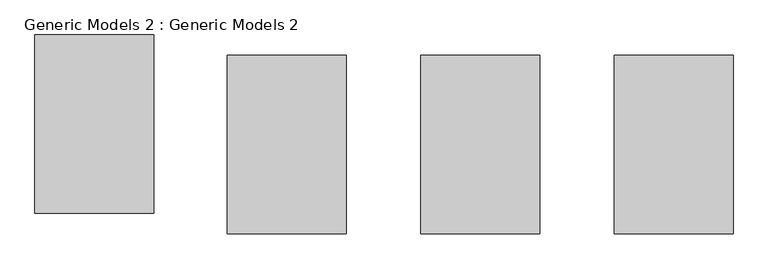
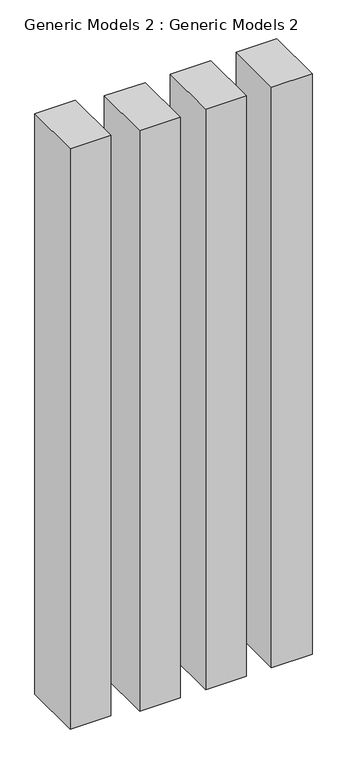
"""IFC4 building model written with IfcOpenShell, lengths in millimetres: proxy geometry, Generic Models 2 : Generic Models 2."""

from ifc_helpers import new_model, si_unit, frame, origin, place, context, project, spatial, polyline, outline, extrude, source, transform, mapped, element, save


def generic_models_2_generic_models_2_13199aed(model_context):
    return source(origin(), model_context, "Body", "SweptSolid", [
        extrude(outline(polyline([(-5406.6672301, -7265.2302427), (-5203.4672301, -7265.2302427), (-5203.4672301, -7570.0302427), (-5406.6672301, -7570.0302427), (-5406.6672301, -7265.2302427)])), frame((0.0, 0.0, 3022.6), z_axis=(0.0, 0.0, 1.0), x_axis=(1.0, 0.0, 0.0)), (0.0, 0.0, 1.0), 3073.4),
        extrude(outline(polyline([(-5736.8672301, -7265.2302427), (-5533.6672301, -7265.2302427), (-5533.6672301, -7570.0302427), (-5736.8672301, -7570.0302427), (-5736.8672301, -7265.2302427)])), frame((0.0, 0.0, 3022.6), z_axis=(0.0, 0.0, 1.0), x_axis=(1.0, 0.0, 0.0)), (0.0, 0.0, 1.0), 3073.4),
        extrude(outline(polyline([(-6067.0672301, -7265.2302427), (-5863.8672301, -7265.2302427), (-5863.8672301, -7570.0302427), (-6067.0672301, -7570.0302427), (-6067.0672301, -7265.2302427)])), frame((0.0, 0.0, 3022.6), z_axis=(0.0, 0.0, 1.0), x_axis=(1.0, 0.0, 0.0)), (0.0, 0.0, 1.0), 3073.4),
        extrude(outline(polyline([(-6395.45836, -7230.7149442), (-6192.25836, -7230.7149442), (-6192.25836, -7535.5149442), (-6395.45836, -7535.5149442), (-6395.45836, -7230.7149442)])), frame((0.0, 0.0, 3022.6), z_axis=(0.0, 0.0, 1.0), x_axis=(1.0, 0.0, 0.0)), (0.0, 0.0, 1.0), 3073.4),
    ])


if __name__ == "__main__":
    model = new_model("IFC4")
    model_context = context("Model", 3, world=origin())
    ifc_project = project(units=[si_unit("LENGTHUNIT", "METRE", prefix="MILLI")], contexts=[model_context])
    site = spatial("IfcSite", under=ifc_project)
    building = spatial("IfcBuilding", under=site)
    placement = place(None, origin())
    generic_models_2_generic_models_2_shape = generic_models_2_generic_models_2_13199aed(model_context)
    element("IfcBuildingElementProxy", 1, Name="Generic Models 2 : Generic Models 2", ObjectType="Generic Models 2 : Generic Models 2", at=placement, inside=building, context=model_context, shape_type="MappedRepresentation", body=[
        mapped(generic_models_2_generic_models_2_shape, transform((0.0, 0.0, 0.0), x_axis=(1.0, 0.0, 0.0), y_axis=(0.0, 1.0, 0.0), z_axis=(0.0, 0.0, 1.0))),
    ])
    save(model, "model.ifc")

# Revit data of these elements
# Element 1 (IfcBuildingElementProxy, "Generic Models 2 : Generic Models 2")
#   Materials on its faces: "MARBLE FLOORING 6\""
# Materials
#   "MARBLE FLOORING 6\"": class "Generic", colour RGB 120 120 120, transparency 0, Cost = 0
